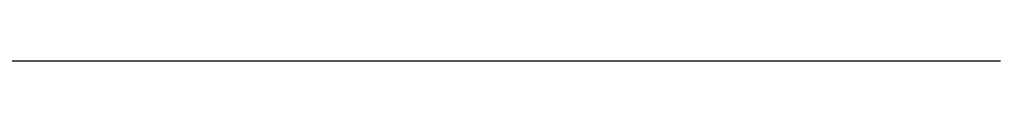
# Model space of a CAD drawing. Units: millimetres. Extents: x 0 to 2267, y 0 to 1823.
# Tile 9 of 256: x 1490.3 to 1505.93, y 1117.32 to 1117.42. Entities that reach past the tile are written whole.
import ezdxf

# ---------------------------------------------------------------- set-up
doc = ezdxf.new("R2010")
doc.units = ezdxf.units.MM
doc.header["$MEASUREMENT"] = 0
doc.layers.add('M-DIMS', color=2, linetype='Continuous', lineweight=25)
doc.styles.get("Standard").update_dxf_attribs({"font": 'arial.ttf'})
doc.dimstyles.get("Standard").update_dxf_attribs({"dimtxt": 7, "dimasz": 4, "dimexe": 0.18, "dimexo": 0.0625, "dimgap": 0.09, "dimtad": 0, "dimdec": 0, "dimzin": 0, "dimdsep": 46, "dimtxsty": 'Standard', "dimcen": 0.09, "dimadec": 0, "dimazin": 0, "dimtfac": 1, "dimtdec": 0, "dimtofl": 0, "dimtmove": 0, "dimatfit": 3, "dimfxl": 1, "dimtolj": 1, "dimtzin": 0, "dimarcsym": 0})

# ---------------------------------------------------------------- blocks, each defined once
blk = doc.blocks.new('*D9')
at = {"layer": 'Defpoints', "color": 0, "transparency": 16777216}
for p in [(1332.087, 1117.417), (1505.929, 1117.417), (1505.929, 1077.417)]:
    blk.add_point(p, dxfattribs=at)
at = {"layer": 'M-DIMS', "color": 0, "lineweight": -2, "transparency": 16777216}
for p, q in [((1505.866, 1117.417), (1331.907, 1117.417)), ((1332.087, 1113.417), (1332.087, 1102.65)), ((1332.087, 1081.417), (1332.087, 1092.184)), ((1505.866, 1077.417), (1331.907, 1077.417))]:
    blk.add_line(p, q, dxfattribs=at)
at = {"layer": 'M-DIMS', "color": 0, "transparency": 16777216}
for points in [[(1331.42, 1113.417), (1332.753, 1113.417), (1332.087, 1117.417)], [(1331.42, 1081.417), (1332.753, 1081.417), (1332.087, 1077.417)]]:
    blk.add_solid(points, dxfattribs=at)
at = {"layer": 'M-DIMS', "color": 0, "transparency": 16777216, "insert": (1332.087, 1097.417), "char_height": 7, "attachment_point": 5, "rotation": 90}
blk.add_mtext('\\A1;40', dxfattribs=at)
blk = doc.blocks.new('*D10')
at = {"layer": 'Defpoints', "color": 0, "transparency": 16777216}
for p in [(1332.087, 1287.766), (1505.929, 1287.766), (1505.929, 1117.417)]:
    blk.add_point(p, dxfattribs=at)
at = {"layer": 'M-DIMS', "color": 0, "lineweight": -2, "transparency": 16777216}
for p, q in [((1505.866, 1287.766), (1331.907, 1287.766)), ((1332.087, 1283.766), (1332.087, 1216.908)), ((1332.087, 1121.417), (1332.087, 1188.275)), ((1505.866, 1117.417), (1331.907, 1117.417))]:
    blk.add_line(p, q, dxfattribs=at)
at = {"layer": 'M-DIMS', "color": 0, "transparency": 16777216}
for points in [[(1331.42, 1283.766), (1332.753, 1283.766), (1332.087, 1287.766)], [(1331.42, 1121.417), (1332.753, 1121.417), (1332.087, 1117.417)]]:
    blk.add_solid(points, dxfattribs=at)
at = {"layer": 'M-DIMS', "color": 0, "transparency": 16777216, "insert": (1332.087, 1202.591), "char_height": 7, "attachment_point": 5, "rotation": 90}
blk.add_mtext('\\A1;170.35', dxfattribs=at)
blk = doc.blocks.new('*D28')
at = {"layer": 'Defpoints', "color": 0, "transparency": 16777216}
for p in [(1523.858, 1124.488), (1530.929, 1117.417)]:
    blk.add_point(p, dxfattribs=at)
at = {"layer": 'M-DIMS', "color": 0, "lineweight": -2, "transparency": 16777216}
for p, q in [((1518.201, 1130.145), (1521.029, 1127.317)), ((1530.929, 1117.327), (1530.929, 1117.507)), ((1530.839, 1117.417), (1531.019, 1117.417))]:
    blk.add_line(p, q, dxfattribs=at)
at = {"layer": 'M-DIMS', "color": 0, "transparency": 16777216}
blk.add_solid([(1521.501, 1127.788), (1520.558, 1126.845), (1523.858, 1124.488)], dxfattribs=at)
at = {"layer": 'M-DIMS', "color": 0, "transparency": 16777216, "insert": (1504.949, 1143.397), "char_height": 7, "attachment_point": 5, "rotation": 314.9998}
blk.add_mtext('\\A1;27X R10', dxfattribs=at)

msp = doc.modelspace()

# ---------------------------------------------------------------- dimensions: what is measured, and where the dimension line sits
at = {"layer": 'M-DIMS'}
for base, p1, p2, override, picture, middle in [((1332.087, 1287.766), (1505.929, 1117.417), (1505.929, 1287.766), {"dimdec": 2, "dimlfac": 1, "dimrnd": 0, "dimzin": 0, "dimdsep": 46, "dimlunit": 2}, '*D10', (1332.087, 1202.591)), ((1332.087, 1117.417), (1505.929, 1077.417), (1505.929, 1117.417), {"dimdec": 0, "dimlfac": 1, "dimrnd": 0, "dimzin": 0, "dimdsep": 46, "dimlunit": 2}, '*D9', (1332.087, 1097.417))]:
    dim = msp.add_linear_dim(base=base, p1=p1, p2=p2, angle=90, dimstyle='Standard', override=override, dxfattribs=at)
    dim.commit()
    dim.dimension.update_dxf_attribs({"geometry": picture, "text_midpoint": middle})
dim = msp.add_radius_dim(center=(1530.929, 1117.417), mpoint=(1523.858, 1124.488), text='27X <>', dimstyle='Standard', override={"dimdec": 0, "dimlfac": 1, "dimrnd": 0, "dimzin": 0, "dimdsep": 46, "dimlunit": 2}, dxfattribs=at)
dim.commit()
dim.dimension.update_dxf_attribs({"geometry": '*D28', "text_midpoint": (1504.949, 1143.397)})

doc.saveas('drawing.dxf')
